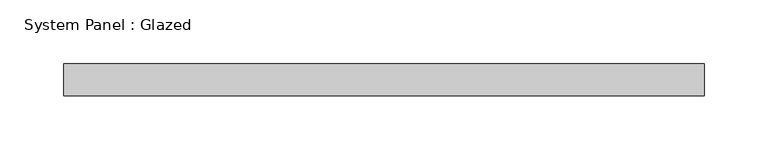
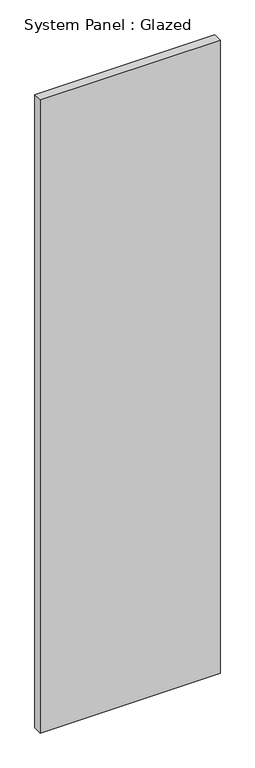
"""IFC4 building model written with IfcOpenShell, lengths in millimetres: plate geometry, System Panel : Glazed."""

from ifc_helpers import new_model, si_unit, origin, origin_with_axes, place, context, project, spatial, polyline, outline, extrude, source, transform, mapped, element, save


def system_panel_glazed_9cdd2f26(model_context):
    return source(origin(), model_context, "Body", "SweptSolid", [
        extrude(outline(polyline([(251.25, 24.5), (-251.25, 24.5), (-251.25, 49.5), (251.25, 49.5), (251.25, 24.5)])), origin_with_axes(), (0.0, 0.0, 1.0), 1870.0),
    ])


if __name__ == "__main__":
    model = new_model("IFC4")
    model_context = context("Model", 3, world=origin())
    ifc_project = project(units=[si_unit("LENGTHUNIT", "METRE", prefix="MILLI")], contexts=[model_context])
    site = spatial("IfcSite", under=ifc_project)
    building = spatial("IfcBuilding", under=site)
    placement = place(None, origin())
    system_panel_glazed_shape = system_panel_glazed_9cdd2f26(model_context)
    element("IfcPlate", 1, ObjectType="System Panel : Glazed", at=placement, inside=building, context=model_context, shape_type="MappedRepresentation", body=[
        mapped(system_panel_glazed_shape, transform((0.0, 0.0, 0.0), x_axis=(1.0, 0.0, 0.0), y_axis=(0.0, 1.0, 0.0), z_axis=(0.0, 0.0, 1.0))),
    ])
    save(model, "model.ifc")

# Revit data of these elements
# Type "System Panel : Glazed"
#   Construction Type Id = "GSP4R"
#   Analytic Construction = "1/8 in Pilkington single glazing"
#   Visual Light Transmittance = 0.9
#   Solar Heat Gain Coefficient = 0.86
#   Heat Transfer Coefficient (U) = 6.7069 W/(m²·K)
#   Define Thermal Properties by = 1
# Element 1 (IfcPlate, "System Panel : Glazed")
#   Materials on its faces: "Glass"
# Materials
#   "Glass": class "Glass", colour RGB 245 245 243, transparency 1, Description = "Soda Lime Glass", Cost = 0
